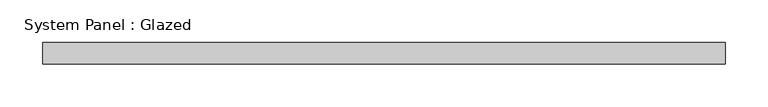
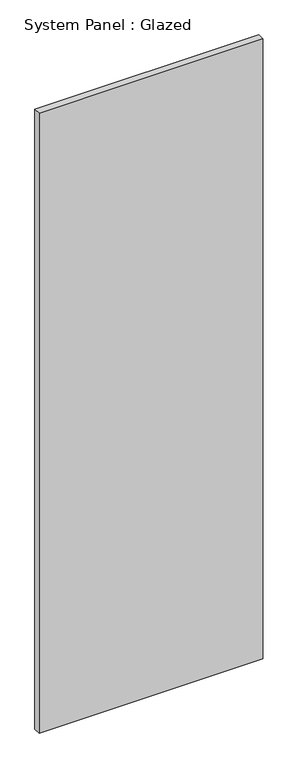
"""IFC4 building model written with IfcOpenShell, lengths in millimetres: plate geometry, System Panel : Glazed."""

from ifc_helpers import new_model, si_unit, origin, origin_with_axes, place, context, project, spatial, polyline, outline, extrude, source, transform, mapped, element, save


def system_panel_glazed_eabd6c1f(model_context):
    return source(origin(), model_context, "Body", "SweptSolid", [
        extrude(outline(polyline([(400.05, 19.05), (-400.05, 19.05), (-400.05, 44.45), (400.05, 44.45), (400.05, 19.05)])), origin_with_axes(), (0.0, 0.0, 1.0), 2341.3449309),
    ])


if __name__ == "__main__":
    model = new_model("IFC4")
    model_context = context("Model", 3, world=origin())
    ifc_project = project(units=[si_unit("LENGTHUNIT", "METRE", prefix="MILLI")], contexts=[model_context])
    site = spatial("IfcSite", under=ifc_project)
    building = spatial("IfcBuilding", under=site)
    placement = place(None, origin())
    system_panel_glazed_shape = system_panel_glazed_eabd6c1f(model_context)
    element("IfcPlate", 1, ObjectType="System Panel : Glazed", at=placement, inside=building, context=model_context, shape_type="MappedRepresentation", body=[
        mapped(system_panel_glazed_shape, transform((0.0, 0.0, 0.0), x_axis=(1.0, 0.0, 0.0), y_axis=(0.0, 1.0, 0.0), z_axis=(0.0, 0.0, 1.0))),
    ])
    save(model, "model.ifc")

# Revit data of these elements
# Type "System Panel : Glazed"
#   Construction Type Id = "GSP4R"
#   Analytic Construction = "1/8 in Pilkington single glazing"
#   Visual Light Transmittance = 0.9
#   Solar Heat Gain Coefficient = 0.86
#   Heat Transfer Coefficient (U) = 1.18115 BTU/(h·ft²·°F)
#   Define Thermal Properties by = 1
# Element 1 (IfcPlate, "System Panel : Glazed")
#   Materials on its faces: "Glass"
# Materials
#   "Glass": class "Glass", colour RGB 0 128 192, transparency 0.75, Description = "Soda Lime Glass", Cost = 0
